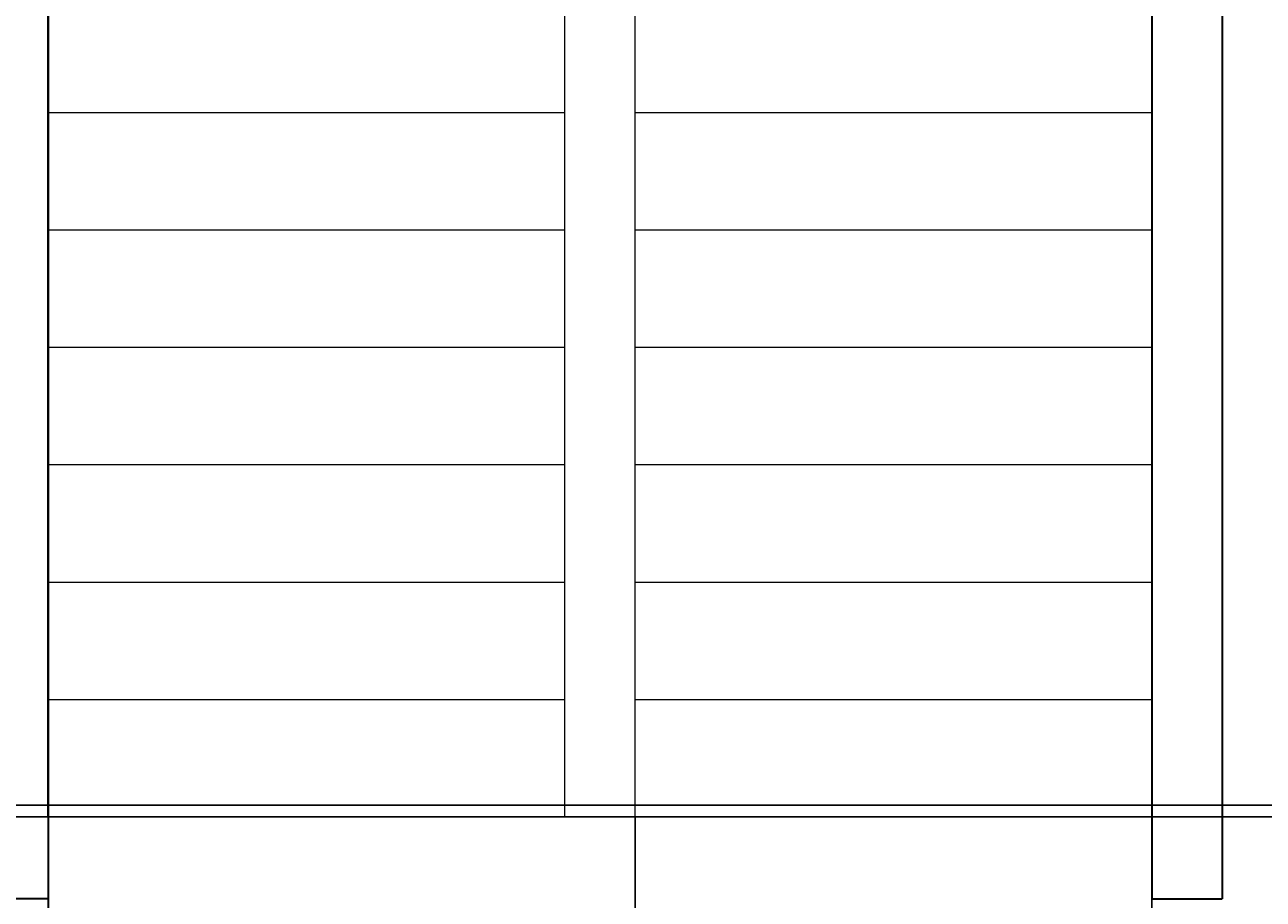
# Model space of a CAD drawing. Units: feet. Extents: x 105 to 1094, y -88 to 588.
# Tile 43 of 59: x 551 to 656, y 288 to 363. Entities that reach past the tile are written whole.
import ezdxf

# ---------------------------------------------------------------- set-up
doc = ezdxf.new("R2010")
doc.units = ezdxf.units.FT
doc.header["$MEASUREMENT"] = 0
for name, color, linetype, lineweight in [('A-ANNO-DIMS', 2, 'Continuous', 18), ('A-FLOR-STRS', 3, 'Continuous', 18), ('A-WALL', 7, 'Continuous', 35)]:
    doc.layers.add(name, color=color, linetype=linetype, lineweight=lineweight)
doc.styles.get("Standard").update_dxf_attribs({"font": 'arial.ttf'})
doc.dimstyles.get("Standard").update_dxf_attribs({"dimtxt": 0.18, "dimasz": 0.18, "dimexe": 0.18, "dimexo": 0.0625, "dimgap": 0.09, "dimtad": 0, "dimtih": 1, "dimtoh": 1, "dimdec": 4, "dimzin": 0, "dimdsep": 46, "dimtxsty": 'Standard', "dimcen": 0.09, "dimadec": 0, "dimazin": 0, "dimtfac": 1, "dimtdec": 4, "dimtofl": 0, "dimtmove": 0, "dimatfit": 3, "dimfxl": 1, "dimtolj": 1, "dimtzin": 0, "dimarcsym": 0})

# ---------------------------------------------------------------- blocks, each defined once
blk = doc.blocks.new('*D21')
at = {"layer": 'A-ANNO-DIMS', "color": 0, "lineweight": -2, "transparency": 16777216}
for p, q in [((849.63, 543.08), (105.46, 543.08)), ((105.64, 542.9), (105.64, 250.26)), ((105.64, -42.74), (105.64, 249.9)), ((849.63, -42.92), (105.46, -42.92))]:
    blk.add_line(p, q, dxfattribs=at)
at = {"layer": 'A-ANNO-DIMS', "color": 0, "transparency": 16777216}
for points in [[(105.61, 542.9), (105.67, 542.9), (105.64, 543.08)], [(105.61, -42.74), (105.67, -42.74), (105.64, -42.92)]]:
    blk.add_solid(points, dxfattribs=at)
at = {"layer": 'Defpoints', "color": 0, "transparency": 16777216}
for p in [(105.64, 543.08), (849.69, 543.08), (849.69, -42.92)]:
    blk.add_point(p, dxfattribs=at)
at = {"layer": 'A-ANNO-DIMS', "color": 0, "transparency": 16777216, "insert": (105.64, 250.08), "char_height": 0.18, "attachment_point": 5}
blk.add_mtext('\\A1;586', dxfattribs=at)
blk = doc.blocks.new('*D33')
at = {"layer": 'A-ANNO-DIMS', "color": 0, "lineweight": -2, "transparency": 16777216}
for p, q in [((646.63, 395.08), (105.46, 395.08)), ((105.64, 394.9), (105.64, 345.26)), ((105.64, 295.26), (105.64, 344.9)), ((646.63, 295.08), (105.46, 295.08))]:
    blk.add_line(p, q, dxfattribs=at)
at = {"layer": 'A-ANNO-DIMS', "color": 0, "transparency": 16777216}
for points in [[(105.61, 394.9), (105.67, 394.9), (105.64, 395.08)], [(105.61, 295.26), (105.67, 295.26), (105.64, 295.08)]]:
    blk.add_solid(points, dxfattribs=at)
at = {"layer": 'Defpoints', "color": 0, "transparency": 16777216}
for p in [(646.69, 395.08), (105.64, 295.08), (646.69, 295.08)]:
    blk.add_point(p, dxfattribs=at)
at = {"layer": 'A-ANNO-DIMS', "color": 0, "transparency": 16777216, "insert": (105.64, 345.08), "char_height": 0.18, "attachment_point": 5}
blk.add_mtext('\\A1;100', dxfattribs=at)
blk = doc.blocks.new('*D34')
at = {"layer": 'A-ANNO-DIMS', "color": 0, "lineweight": -2, "transparency": 16777216}
for p, q in [((552.75, 295.08), (1093.92, 295.08)), ((1093.74, 294.9), (1093.74, 253.76)), ((1093.74, 212.26), (1093.74, 253.4)), ((552.75, 212.08), (1093.92, 212.08))]:
    blk.add_line(p, q, dxfattribs=at)
at = {"layer": 'A-ANNO-DIMS', "color": 0, "transparency": 16777216}
for points in [[(1093.71, 294.9), (1093.77, 294.9), (1093.74, 295.08)], [(1093.71, 212.26), (1093.77, 212.26), (1093.74, 212.08)]]:
    blk.add_solid(points, dxfattribs=at)
at = {"layer": 'Defpoints', "color": 0, "transparency": 16777216}
for p in [(552.69, 295.08), (552.69, 212.08), (1093.74, 212.08)]:
    blk.add_point(p, dxfattribs=at)
at = {"layer": 'A-ANNO-DIMS', "color": 0, "transparency": 16777216, "insert": (1093.74, 253.58), "char_height": 0.18, "attachment_point": 5}
blk.add_mtext('\\A1;83', dxfattribs=at)
blk = doc.blocks.new('*D49')
at = {"layer": 'A-ANNO-DIMS', "color": 0, "lineweight": -2, "transparency": 16777216}
for p, q in [((602.69, 295.02), (602.69, -88.15)), ((646.69, 295.02), (646.69, -88.15)), ((602.87, -87.97), (624.47, -87.97)), ((646.51, -87.97), (624.91, -87.97))]:
    blk.add_line(p, q, dxfattribs=at)
at = {"layer": 'A-ANNO-DIMS', "color": 0, "transparency": 16777216}
for points in [[(602.87, -87.94), (602.87, -88), (602.69, -87.97)], [(646.51, -87.94), (646.51, -88), (646.69, -87.97)]]:
    blk.add_solid(points, dxfattribs=at)
at = {"layer": 'Defpoints', "color": 0, "transparency": 16777216}
for p in [(602.69, 295.08), (646.69, 295.08), (646.69, -87.97)]:
    blk.add_point(p, dxfattribs=at)
at = {"layer": 'A-ANNO-DIMS', "color": 0, "transparency": 16777216, "insert": (624.69, -87.97), "char_height": 0.18, "attachment_point": 5}
blk.add_mtext('\\A1;44', dxfattribs=at)
blk = doc.blocks.new('*D54')
at = {"layer": 'A-ANNO-DIMS', "color": 0, "lineweight": -2, "transparency": 16777216}
for p, q in [((294.75, 296.08), (1093.92, 296.08)), ((1093.74, 295.9), (1093.74, 286.26)), ((1093.74, 276.26), (1093.74, 285.9)), ((294.75, 276.08), (1093.92, 276.08))]:
    blk.add_line(p, q, dxfattribs=at)
at = {"layer": 'A-ANNO-DIMS', "color": 0, "transparency": 16777216}
for points in [[(1093.71, 295.9), (1093.77, 295.9), (1093.74, 296.08)], [(1093.71, 276.26), (1093.77, 276.26), (1093.74, 276.08)]]:
    blk.add_solid(points, dxfattribs=at)
at = {"layer": 'Defpoints', "color": 0, "transparency": 16777216}
for p in [(294.69, 296.08), (1093.74, 296.08), (294.69, 276.08)]:
    blk.add_point(p, dxfattribs=at)
at = {"layer": 'A-ANNO-DIMS', "color": 0, "transparency": 16777216, "insert": (1093.74, 286.08), "char_height": 0.18, "attachment_point": 5}
blk.add_mtext('\\A1;20', dxfattribs=at)

msp = doc.modelspace()

# ---------------------------------------------------------------- linework, layer by layer
at = {"layer": 'A-FLOR-STRS'}
for p, q in [((596.6883, 295.0812), (596.6883, 395.0812)), ((602.6883, 295.0812), (602.6883, 395.0812)), ((552.6883, 355.0812), (596.6883, 355.0812)), ((602.6883, 355.0812), (646.6883, 355.0812)), ((552.6883, 345.0812), (596.6883, 345.0812)), ((602.6883, 345.0812), (646.6883, 345.0812)), ((552.6883, 335.0812), (596.6883, 335.0812)), ((602.6883, 335.0812), (646.6883, 335.0812)), ((552.6883, 325.0812), (596.6883, 325.0812)), ((602.6883, 325.0812), (646.6883, 325.0812)), ((552.6883, 315.0812), (596.6883, 315.0812)), ((602.6883, 315.0812), (646.6883, 315.0812)), ((552.6883, 305.0812), (596.6883, 305.0812)), ((602.6883, 305.0812), (646.6883, 305.0812)), ((552.6883, 295.0812), (646.6883, 295.0812))]:
    msp.add_line(p, q, dxfattribs=at)
at = {"layer": 'A-WALL'}
for p, q in [((552.6883, 295.0812), (552.6883, 441.0812)), ((552.6883, 441.0812), (552.6883, 288.0812)), ((646.6883, 441.0812), (646.6883, 288.0812)), ((652.6883, 435.0812), (652.6883, 288.0812)), ((552.6883, 295.0812), (552.6883, 206.0812)), ((552.6883, 288.0812), (546.6883, 288.0812)), ((646.6883, 288.0812), (652.6883, 288.0812))]:
    msp.add_line(p, q, dxfattribs=at)

# ---------------------------------------------------------------- dimensions: what is measured, and where the dimension line sits
at = {"layer": 'A-ANNO-DIMS'}
for base, p1, p2, picture, middle in [((105.6383, 543.0812), (849.6883, -42.9188), (849.6883, 543.0812), '*D21', (105.6383, 250.0812)), ((105.6383, 295.0812), (646.6883, 395.0812), (646.6883, 295.0812), '*D33', (105.6383, 345.0812)), ((1093.7383, 296.0812), (294.6883, 276.0812), (294.6883, 296.0812), '*D54', (1093.7383, 286.0812)), ((1093.7383, 212.0812), (552.6883, 295.0812), (552.6883, 212.0812), '*D34', (1093.7383, 253.5812))]:
    dim = msp.add_linear_dim(base=base, p1=p1, p2=p2, angle=90, dimstyle='Standard', override={"dimdec": 0, "dimlfac": 1, "dimrnd": 0, "dimzin": 0, "dimdsep": 46, "dimlunit": 2}, dxfattribs=at)
    dim.commit()
    dim.dimension.update_dxf_attribs({"geometry": picture, "text_midpoint": middle})
dim = msp.add_linear_dim(base=(646.6883, -87.9688), p1=(602.6883, 295.0812), p2=(646.6883, 295.0812), dimstyle='Standard', override={"dimdec": 0, "dimlfac": 1, "dimrnd": 0, "dimzin": 0, "dimdsep": 46, "dimlunit": 2}, dxfattribs=at)
dim.commit()
dim.dimension.update_dxf_attribs({"geometry": '*D49', "text_midpoint": (624.6883, -87.9688)})

doc.saveas('drawing.dxf')
